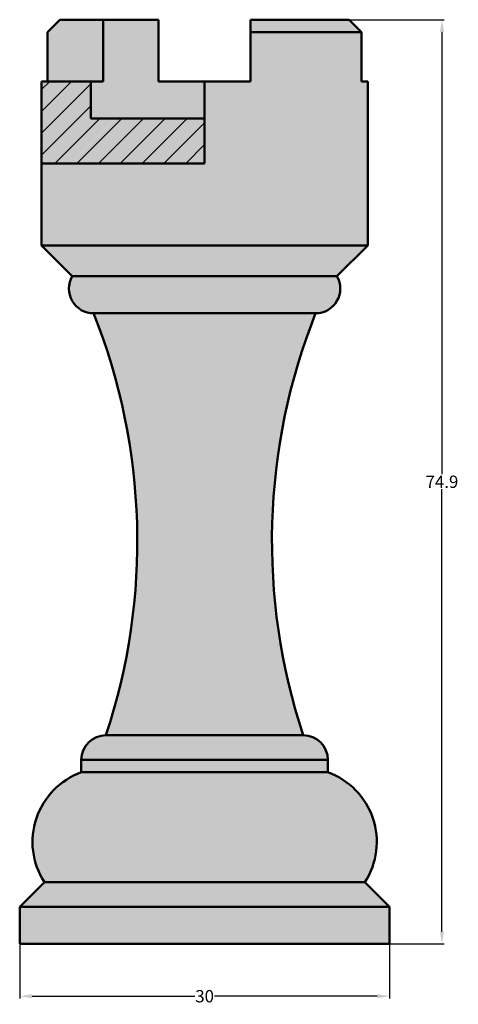
# Model space of a CAD drawing. Units: millimetres. Extents: x 31 to 232, y 35 to 192.
# Tile 5 of 5: x 197 to 232, y 39 to 119. Entities that reach past the tile are written whole.
import ezdxf

# ---------------------------------------------------------------- set-up
doc = ezdxf.new("R2010")
doc.units = ezdxf.units.MM
doc.header["$MEASUREMENT"] = 0
for name, color, linetype, lineweight in [('M-DIMS', 2, 'Continuous', 25), ('M-HATC', 8, 'Continuous', 18), ('M-OUTL', 7, 'Continuous', 50)]:
    doc.layers.add(name, color=color, linetype=linetype, lineweight=lineweight)
doc.styles.get("Standard").update_dxf_attribs({"font": 'arial.ttf'})
doc.dimstyles.get("Standard").update_dxf_attribs({"dimtxt": 1, "dimasz": 1, "dimexe": 0.18, "dimexo": 0.0625, "dimgap": 0.09, "dimtad": 0, "dimtih": 1, "dimtoh": 1, "dimdec": 0, "dimzin": 0, "dimdsep": 46, "dimtxsty": 'Standard', "dimcen": 0.09, "dimadec": 0, "dimazin": 0, "dimtfac": 1, "dimtdec": 0, "dimtofl": 0, "dimtmove": 0, "dimatfit": 3, "dimfxl": 1, "dimtolj": 1, "dimtzin": 0, "dimarcsym": 0})

# ---------------------------------------------------------------- blocks, each defined once
blk = doc.blocks.new('*D45')
at = {"layer": 'Defpoints', "color": 0, "transparency": 16777216}
for p in [(196.716, 44.153), (226.716, 44.153), (226.716, 39.903)]:
    blk.add_point(p, dxfattribs=at)
at = {"layer": 'M-DIMS', "color": 0, "lineweight": -2, "transparency": 16777216}
for p, q in [((196.716, 44.091), (196.716, 39.723)), ((226.716, 44.091), (226.716, 39.723)), ((197.716, 39.903), (210.912, 39.903)), ((225.716, 39.903), (212.52, 39.903))]:
    blk.add_line(p, q, dxfattribs=at)
at = {"layer": 'M-DIMS', "color": 0, "transparency": 16777216}
for points in [[(197.716, 40.07), (197.716, 39.737), (196.716, 39.903)], [(225.716, 40.07), (225.716, 39.737), (226.716, 39.903)]]:
    blk.add_solid(points, dxfattribs=at)
at = {"layer": 'M-DIMS', "color": 0, "transparency": 16777216, "insert": (211.716, 39.903), "char_height": 1, "attachment_point": 5}
blk.add_mtext('\\A1;30', dxfattribs=at)
blk = doc.blocks.new('*D46')
at = {"layer": 'Defpoints', "color": 0, "transparency": 16777216}
for p in [(215.448, 119.053), (230.966, 119.053), (196.716, 44.153)]:
    blk.add_point(p, dxfattribs=at)
at = {"layer": 'M-DIMS', "color": 0, "lineweight": -2, "transparency": 16777216}
for p, q in [((215.511, 119.053), (231.146, 119.053)), ((230.966, 118.053), (230.966, 82.204)), ((230.966, 45.153), (230.966, 81.003)), ((196.779, 44.153), (231.146, 44.153))]:
    blk.add_line(p, q, dxfattribs=at)
at = {"layer": 'M-DIMS', "color": 0, "transparency": 16777216}
for points in [[(230.8, 118.053), (231.133, 118.053), (230.966, 119.053)], [(230.8, 45.153), (231.133, 45.153), (230.966, 44.153)]]:
    blk.add_solid(points, dxfattribs=at)
at = {"layer": 'M-DIMS', "color": 0, "transparency": 16777216, "insert": (230.966, 81.603), "char_height": 1, "attachment_point": 5}
blk.add_mtext('\\A1;74.9', dxfattribs=at)

msp = doc.modelspace()

# ---------------------------------------------------------------- hatches: boundary and pattern name
at = {"layer": 'M-HATC'}
h = msp.add_hatch(color=256, dxfattribs=at)
h.dxf.hatch_style = 1
h.paths.add_polyline_path([(221.7162, 58.0533), (211.7162, 58.0533), (201.7162, 58.0533, 0.4824021), (198.7162, 49.1533), (211.7162, 49.1533), (224.7162, 49.1533, 0.4824021)])
h.paths.add_polyline_path([(226.7162, 47.1533), (196.7162, 47.1533), (196.7162, 44.1533), (226.7162, 44.1533)])
h.paths.add_polyline_path([(224.7162, 49.1533), (211.7162, 49.1533), (198.7162, 49.1533), (196.7162, 47.1533), (226.7162, 47.1533)])
h.paths.add_polyline_path([(219.7162, 61.0533), (211.7162, 61.0533), (203.7162, 61.0533, 0.4142136), (201.7162, 59.0533), (211.7162, 59.0533), (221.7162, 59.0533, 0.4142136)])
h.paths.add_polyline_path([(221.7162, 59.0533), (211.7162, 59.0533), (201.7162, 59.0533), (201.7162, 58.0533), (211.7162, 58.0533), (221.7162, 58.0533)])
h.paths.add_polyline_path([(220.7162, 95.2533), (211.7162, 95.2533), (202.7162, 95.2533, -0.1763961), (203.7162, 61.0533), (211.7162, 61.0533), (219.7162, 61.0533, -0.1763961)])
h.paths.add_polyline_path([(222.4483, 98.2533), (213.4483, 98.2533), (211.7162, 98.2533), (209.9842, 98.2533), (200.9842, 98.2533, 0.5773503), (202.7162, 95.2533), (211.7162, 95.2533), (220.7162, 95.2533, 0.5773503)])
h.paths.add_polyline_path([(224.9483, 100.7533), (211.7162, 100.7533), (198.4842, 100.7533), (200.9842, 98.2533), (209.9842, 98.2533), (211.7162, 98.2533), (213.4483, 98.2533), (222.4483, 98.2533)])
h.paths.add_polyline_path([(224.9483, 114.0533), (224.4483, 114.0533), (224.4483, 118.0533), (215.4483, 118.0533), (215.4483, 114.0533), (211.7162, 114.0533), (211.7162, 111.0533), (211.7162, 107.4033), (198.4842, 107.4033), (198.4842, 100.7533), (211.7162, 100.7533), (224.9483, 100.7533)])
h.paths.add_polyline_path([(223.4483, 119.0533), (215.4483, 119.0533), (215.4483, 118.0533), (224.4483, 118.0533)])
h.paths.add_polyline_path([(211.7162, 111.0533), (202.4842, 111.0533), (202.4842, 114.0533), (198.4842, 114.0533), (198.4842, 107.4033), (211.7162, 107.4033)], flags=17)
h.paths.add_polyline_path([(211.7162, 114.0533), (207.9842, 114.0533), (207.9842, 119.0533), (203.4842, 119.0533), (203.4842, 114.0533), (202.4842, 114.0533), (202.4842, 111.0533), (211.7162, 111.0533)])
h.paths.add_polyline_path([(203.4842, 119.0533), (199.9842, 119.0533), (198.9842, 118.0533), (198.9842, 114.0533), (202.4842, 114.0533), (203.4842, 114.0533)])
h = msp.add_hatch(dxfattribs=at)
h.set_pattern_fill('ANSI31', color=256, scale=10)
h.set_pattern_definition([(45, (147.9426, 0.9704), (-0.883883, 0.883883), [])])
h.paths.add_polyline_path([(211.7162, 111.0533), (202.4842, 111.0533), (202.4842, 114.0533), (198.4842, 114.0533), (198.4842, 107.4033), (211.7162, 107.4033)])

# ---------------------------------------------------------------- linework, layer by layer
at = {"layer": 'M-OUTL'}
for p, q in [((198.9842, 118.0533), (199.9842, 119.0533)), ((199.9842, 119.0533), (207.9842, 119.0533)), ((203.4842, 114.0533), (203.4842, 119.0533)), ((207.9842, 119.0533), (207.9842, 114.0533)), ((223.4483, 119.0533), (215.4483, 119.0533)), ((215.4483, 119.0533), (215.4483, 114.0533)), ((224.4483, 118.0533), (223.4483, 119.0533)), ((198.9842, 114.0533), (198.9842, 118.0533)), ((224.4483, 118.0533), (215.4483, 118.0533)), ((224.4483, 114.0533), (224.4483, 118.0533)), ((198.4842, 114.0533), (198.4842, 100.7533)), ((198.4842, 114.0533), (202.4842, 114.0533)), ((202.4842, 114.0533), (202.4842, 111.0533)), ((202.4842, 114.0533), (203.4842, 114.0533)), ((207.9842, 114.0533), (211.7162, 114.0533)), ((215.4483, 114.0533), (211.7162, 114.0533)), ((211.7162, 111.0533), (211.7162, 114.0533)), ((224.9483, 114.0533), (224.4483, 114.0533)), ((224.9483, 114.0533), (224.4483, 114.0533)), ((224.9483, 114.0533), (224.4483, 114.0533)), ((224.9483, 114.0533), (224.9483, 100.7533)), ((202.4842, 111.0533), (211.7162, 111.0533)), ((211.7162, 111.0533), (211.7162, 107.4033)), ((211.7162, 111.0533), (211.7162, 107.4033)), ((211.7162, 107.4033), (198.4842, 107.4033)), ((200.9842, 98.2533), (198.4842, 100.7533)), ((198.4842, 100.7533), (211.7162, 100.7533)), ((224.9483, 100.7533), (211.7162, 100.7533)), ((222.4483, 98.2533), (224.9483, 100.7533)), ((200.9842, 98.2533), (209.9842, 98.2533)), ((209.9842, 98.2533), (211.7162, 98.2533)), ((213.4483, 98.2533), (211.7162, 98.2533)), ((222.4483, 98.2533), (213.4483, 98.2533)), ((202.7162, 95.2533), (211.7162, 95.2533)), ((211.7162, 95.2533), (220.7162, 95.2533)), ((203.7162, 61.0533), (211.7162, 61.0533)), ((219.7162, 61.0533), (211.7162, 61.0533)), ((201.7162, 59.0533), (211.7162, 59.0533)), ((201.7162, 59.0533), (201.7162, 58.0533)), ((221.7162, 59.0533), (211.7162, 59.0533)), ((221.7162, 59.0533), (221.7162, 58.0533)), ((211.7162, 58.0533), (201.7162, 58.0533)), ((211.7162, 58.0533), (221.7162, 58.0533)), ((198.7162, 49.1533), (196.7162, 47.1533)), ((211.7162, 49.1533), (198.7162, 49.1533)), ((211.7162, 49.1533), (224.7162, 49.1533)), ((224.7162, 49.1533), (226.7162, 47.1533)), ((226.7162, 47.1533), (196.7162, 47.1533)), ((196.7162, 47.1533), (196.7162, 44.1533)), ((226.7162, 44.1533), (226.7162, 47.1533)), ((196.7162, 44.1533), (226.7162, 44.1533))]:
    msp.add_line(p, q, dxfattribs=at)
for centre, radius, start, end in [((202.7162, 97.2533), 2, 150, 270), ((220.7162, 97.2533), 2, 270, 30), ((156.2539, 76.7801), 50, 341.667154, 21.682522), ((267.1785, 76.7801), 50, 158.317478, 198.332846), ((203.7162, 59.0533), 2, 90, 180), ((219.7162, 59.0533), 2, 0, 90), ((203.7552, 52.4103), 6, 109.866614, 212.87766), ((219.6772, 52.4103), 6, 327.12234, 70.133386)]:
    msp.add_arc(centre, radius, start, end, dxfattribs=at)

# ---------------------------------------------------------------- dimensions: what is measured, and where the dimension line sits
at = {"layer": 'M-DIMS'}
dim = msp.add_linear_dim(base=(230.9662, 119.0533), p1=(196.7162, 44.1533), p2=(215.4483, 119.0533), angle=90, dimstyle='Standard', override={"dimdec": 1, "dimlfac": 1, "dimrnd": 0, "dimzin": 0, "dimdsep": 46, "dimlunit": 2}, dxfattribs=at)
dim.commit()
dim.dimension.update_dxf_attribs({"geometry": '*D46', "text_midpoint": (230.9662, 81.6033)})
dim = msp.add_linear_dim(base=(226.7162, 39.9033), p1=(196.7162, 44.1533), p2=(226.7162, 44.1533), dimstyle='Standard', override={"dimdec": 0, "dimlfac": 1, "dimrnd": 0, "dimzin": 0, "dimdsep": 46, "dimlunit": 2}, dxfattribs=at)
dim.commit()
dim.dimension.update_dxf_attribs({"geometry": '*D45', "text_midpoint": (211.7162, 39.9033)})

doc.saveas('drawing.dxf')
